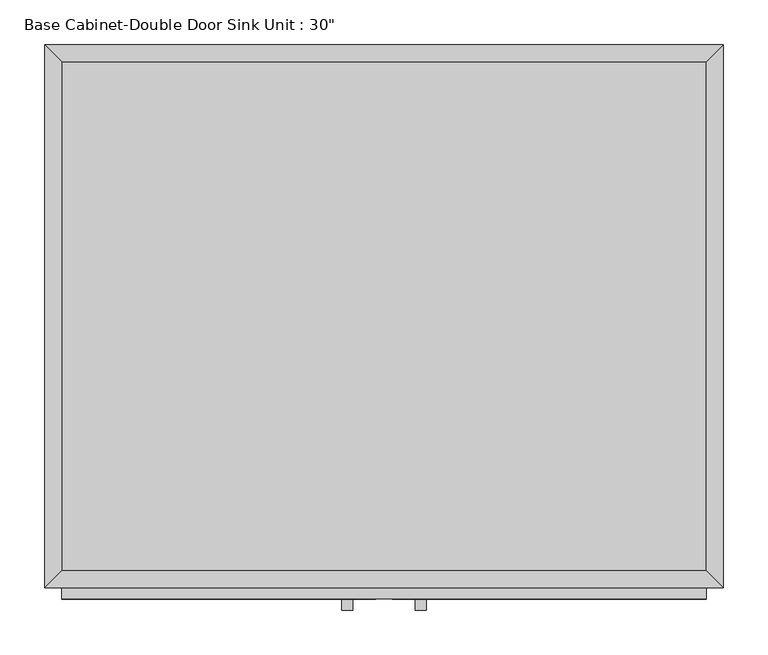
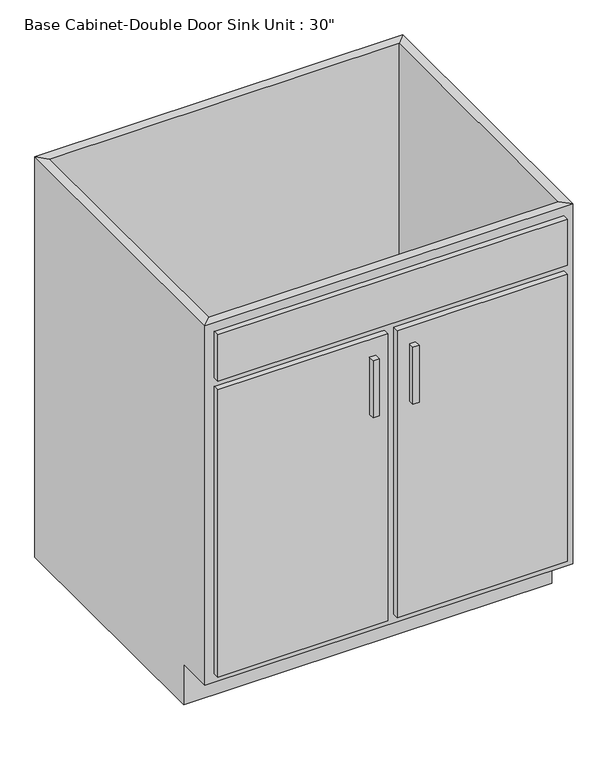
"""IFC4 building model written with IfcOpenShell, lengths in millimetres: furniture geometry."""

from ifc_helpers import new_model, si_unit, frame, origin, place, context, project, spatial, polyline, outline, extrude, faceted_brep, source, transform, mapped, element, save


def furniture_5bfe328f(model_context):
    return source(origin(), model_context, "Body", "SolidModel", [
        faceted_brep([(380.6877049, -590.55, 876.3), (380.6877049, -590.55, 88.9), (-343.2122951, -590.55, 88.9), (-343.2122951, -590.55, 876.3), (-362.2622951, -609.6, 876.3), (399.7377049, -609.6, 876.3), (-362.2622951, -609.6, 88.9), (399.7377049, -609.6, 88.9), (-343.2122951, -533.4, 88.9), (-343.2122951, -19.05, 88.9), (-343.2122951, -19.05, 876.3), (-362.2622951, 0.0, 876.3), (-362.2622951, 0.0, 0.0), (-362.2622951, -533.4, 0.0), (-362.2622951, -533.4, 88.9), (380.6877049, -19.05, 88.9), (380.6877049, -19.05, 876.3), (399.7377049, 0.0, 876.3), (399.7377049, 0.0, 0.0), (380.6877049, -533.4, 88.9), (399.7377049, -533.4, 88.9), (399.7377049, -533.4, 0.0)], [[[0, 1, 2, 3]], [[0, 3, 4, 5]], [[5, 4, 6, 7]], [[2, 1, 7, 6]], [[3, 2, 8, 9, 10]], [[4, 3, 10, 11]], [[6, 4, 11, 12, 13, 14]], [[2, 6, 14, 8]], [[10, 9, 15, 16]], [[11, 10, 16, 17]], [[12, 11, 17, 18]], [[1, 0, 16, 15, 19]], [[0, 5, 17, 16]], [[5, 7, 20, 21, 18, 17]], [[7, 1, 19, 20]], [[8, 19, 15, 9]], [[18, 21, 13, 12]], [[13, 21, 20, 19, 8, 14]]]),
        extrude(outline(polyline([(-16.1872951, -635.0), (-28.8872951, -635.0), (-28.8872951, -622.3), (-16.1872951, -622.3), (-16.1872951, -635.0)])), frame((0.0, 0.0, 573.769895), z_axis=(0.0, 0.0, 1.0), x_axis=(1.0, 0.0, 0.0)), (0.0, 0.0, 1.0), 124.730105),
        extrude(outline(polyline([(66.3627049, -635.0), (53.6627049, -635.0), (53.6627049, -622.3), (66.3627049, -622.3), (66.3627049, -635.0)])), frame((0.0, 0.0, 573.769895), z_axis=(0.0, 0.0, 1.0), x_axis=(1.0, 0.0, 0.0)), (0.0, 0.0, 1.0), 124.730105),
        extrude(outline(polyline([(380.6877049, -19.05), (380.6877049, -590.55), (-343.2122951, -590.55), (-343.2122951, -19.05), (380.6877049, -19.05)])), frame((0.0, 0.0, 88.9), z_axis=(0.0, 0.0, 1.0), x_axis=(1.0, 0.0, 0.0)), (0.0, 0.0, 1.0), 19.05),
        extrude(outline(polyline([(9.2127049, -622.3), (-343.2122951, -622.3), (-343.2122951, -609.6), (9.2127049, -609.6), (9.2127049, -622.3)])), frame((0.0, 0.0, 107.95), z_axis=(0.0, 0.0, 1.0), x_axis=(1.0, 0.0, 0.0)), (0.0, 0.0, 1.0), 628.65),
        extrude(outline(polyline([(380.6877049, -622.3), (28.2627049, -622.3), (28.2627049, -609.6), (380.6877049, -609.6), (380.6877049, -622.3)])), frame((0.0, 0.0, 107.95), z_axis=(0.0, 0.0, 1.0), x_axis=(1.0, 0.0, 0.0)), (0.0, 0.0, 1.0), 628.65),
        extrude(outline(polyline([(380.6877049, -622.3), (-343.2122951, -622.3), (-343.2122951, -609.6), (380.6877049, -609.6), (380.6877049, -622.3)])), frame((0.0, 0.0, 755.65), z_axis=(0.0, 0.0, 1.0), x_axis=(1.0, 0.0, 0.0)), (0.0, 0.0, 1.0), 101.6),
    ])


if __name__ == "__main__":
    model = new_model("IFC4")
    model_context = context("Model", 3, world=origin())
    ifc_project = project(units=[si_unit("LENGTHUNIT", "METRE", prefix="MILLI")], contexts=[model_context])
    site = spatial("IfcSite", under=ifc_project)
    building = spatial("IfcBuilding", under=site)
    placement = place(None, origin())
    furniture_shape = furniture_5bfe328f(model_context)
    element("IfcFurniture", 1, ObjectType="Base Cabinet-Double Door Sink Unit : 30\"", at=placement, inside=building, context=model_context, shape_type="MappedRepresentation", body=[
        mapped(furniture_shape, transform((0.0, 0.0, 0.0), x_axis=(1.0, 0.0, 0.0), y_axis=(0.0, 1.0, 0.0), z_axis=(0.0, 0.0, 1.0))),
    ])
    save(model, "model.ifc")

# Revit data of these elements
# Type "Base Cabinet-Double Door Sink Unit : 30\""
#   Assembly Code = "C1030410"
#   Depth = 2' - 0"
#   Height = 2' - 10 1/2"
#   Toe Depth = 0' - 3"
#   Toe Height = 0' - 3 1/2"
#   Width = 2' - 6"
#   Cabinet Material = none
#   Door/Drawer Material = none
#   Handle Material = Cabinets - Handles
#   Default Elevation = 0
# Element 1 (IfcFurniture, "Base Cabinet-Double Door Sink Unit : 30\"")
#   Materials on its faces: "Cabinets", "Cabinets - Handles"
# Materials
#   "Cabinets - Handles": class "Metal", colour RGB 57 57 57, transparency 0
#   "Cabinets": colour RGB 249 249 249, transparency 0
